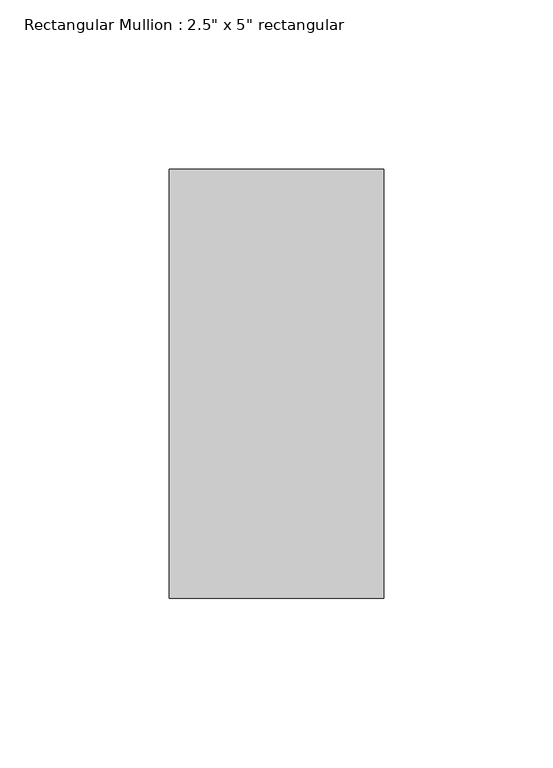
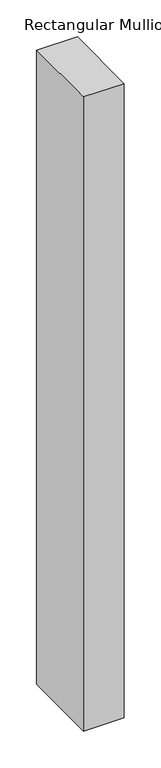
"""IFC4 building model written with IfcOpenShell, lengths in millimetres: member geometry."""

from ifc_helpers import new_model, si_unit, frame, origin, place, context, project, spatial, polyline, outline, extrude, source, transform, mapped, element, save


def member_78934672(model_context):
    return source(origin(), model_context, "Body", "SweptSolid", [
        extrude(outline(polyline([(0.0, 63.5), (0.0, -63.5), (-63.5, -63.5), (-63.5, 63.5), (0.0, 63.5)])), frame((0.0, 0.0, -1047.75), z_axis=(0.0, 0.0, 1.0), x_axis=(1.0, 0.0, 0.0)), (0.0, 0.0, 1.0), 1047.75),
    ])


if __name__ == "__main__":
    model = new_model("IFC4")
    model_context = context("Model", 3, world=origin())
    ifc_project = project(units=[si_unit("LENGTHUNIT", "METRE", prefix="MILLI")], contexts=[model_context])
    site = spatial("IfcSite", under=ifc_project)
    building = spatial("IfcBuilding", under=site)
    placement = place(None, origin())
    member_shape = member_78934672(model_context)
    element("IfcMember", 1, ObjectType="Rectangular Mullion : 2.5\" x 5\" rectangular", at=placement, inside=building, context=model_context, shape_type="MappedRepresentation", body=[
        mapped(member_shape, transform((0.0, 0.0, 0.0), x_axis=(1.0, 0.0, 0.0), y_axis=(0.0, 1.0, 0.0), z_axis=(0.0, 0.0, 1.0))),
    ])
    save(model, "model.ifc")

# Revit data of these elements
# Type "Rectangular Mullion : 2.5\" x 5\" rectangular"
#   built-in parameter 1007304 = 0.416667 (stored number, unit not read)
#   built-in parameter 1007301 = 0.104167 (stored number, unit not read)
#   built-in parameter 1007300 = 0.104167 (stored number, unit not read)
# Element 1 (IfcMember, "Rectangular Mullion : 2.5\" x 5\" rectangular")
#   Materials on its faces: "Aluminum"
# Materials
#   "Aluminum": class "Metal", colour RGB 247 247 247, transparency 0, Description = "Aluminum 6061", Cost = 0
